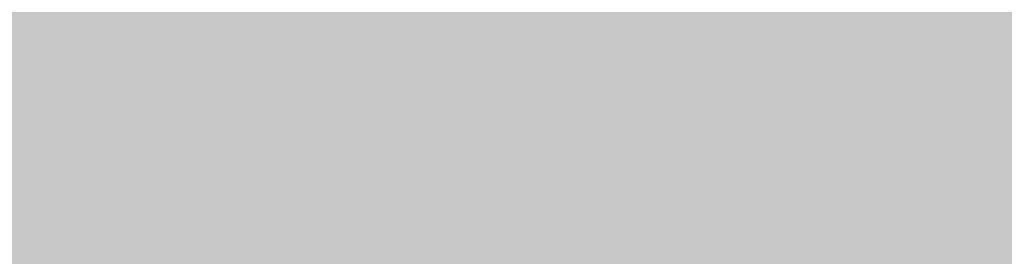
# Model space of a CAD drawing. Units: inches. Extents: x 2083 to 3317, y 1141 to 2115.
# Tile 135 of 256: x 3123.979 to 3126.132, y 1263.613 to 1264.131. Entities that reach past the tile are written whole.
import ezdxf

# ---------------------------------------------------------------- set-up
doc = ezdxf.new("R2010")
doc.units = ezdxf.units.IN
doc.layers.add('A-ANNO-DIMS', color=2, linetype='Continuous', lineweight=18)
doc.layers.add('A-WALL-PATT', color=251, linetype='Continuous', lineweight=13, true_color=0x636466)
doc.styles.get("Standard").update_dxf_attribs({"font": 'arial.ttf'})
doc.dimstyles.new('ISO-25', dxfattribs={"dimtxt": 12, "dimasz": 12, "dimexe": 1.25, "dimexo": 0.625, "dimtad": 1, "dimlunit": 3, "dimtxsty": 'Standard', "dimcen": 2.5, "dimadec": 0, "dimazin": 0, "dimtfac": 1, "dimtmove": 0, "dimatfit": 3, "dimfxl": 1, "dimarcsym": 0})

# ---------------------------------------------------------------- blocks, each defined once
blk = doc.blocks.new('*D26')
at = {"layer": 'A-ANNO-DIMS', "color": 0, "lineweight": -2, "transparency": 16777216}
for p, q in [((3088.9858, 1274.9151), (3088.9858, 1270.952)), ((3111.24, 1274.9151), (3111.24, 1270.952)), ((3076.9858, 1272.202), (2840.2624, 1272.202)), ((3111.24, 1272.202), (3088.9858, 1272.202)), ((3123.24, 1272.202), (3135.24, 1272.202))]:
    blk.add_line(p, q, dxfattribs=at)
at = {"layer": 'A-ANNO-DIMS', "color": 0, "transparency": 16777216}
for points in [[(3076.9858, 1274.202), (3076.9858, 1270.202), (3088.9858, 1272.202)], [(3123.24, 1274.202), (3123.24, 1270.202), (3111.24, 1272.202)]]:
    blk.add_solid(points, dxfattribs=at)
at = {"layer": 'Defpoints', "color": 0, "transparency": 16777216}
for p in [(3088.9858, 1275.5401), (3111.24, 1275.5401), (3088.9858, 1272.202)]:
    blk.add_point(p, dxfattribs=at)
at = {"layer": 'A-ANNO-DIMS', "color": 0, "transparency": 16777216, "insert": (2952.6241, 1279.0316), "char_height": 12, "attachment_point": 5}
blk.add_mtext('NIGHTSTAND 1\'-10 1/2" TYP.', dxfattribs=at)
blk = doc.blocks.new('*D27')
at = {"layer": 'A-ANNO-DIMS', "color": 0, "lineweight": -2, "transparency": 16777216}
for p, q in [((3114.5782, 1309.7943), (3114.5782, 1321.7943)), ((3111.865, 1297.7943), (3115.8282, 1297.7943)), ((3114.5782, 1297.7943), (3114.5782, 1275.5401)), ((3111.865, 1275.5401), (3115.8282, 1275.5401)), ((3114.5782, 1263.5401), (3114.5782, 1140.9886))]:
    blk.add_line(p, q, dxfattribs=at)
at = {"layer": 'A-ANNO-DIMS', "color": 0, "transparency": 16777216}
for points in [[(3112.5782, 1309.7943), (3116.5782, 1309.7943), (3114.5782, 1297.7943)], [(3112.5782, 1263.5401), (3116.5782, 1263.5401), (3114.5782, 1275.5401)]]:
    blk.add_solid(points, dxfattribs=at)
at = {"layer": 'Defpoints', "color": 0, "transparency": 16777216}
for p in [(3111.24, 1297.7943), (3111.24, 1275.5401), (3114.5782, 1275.5401)]:
    blk.add_point(p, dxfattribs=at)
at = {"layer": 'A-ANNO-DIMS', "color": 0, "transparency": 16777216, "insert": (3107.7485, 1196.2643), "char_height": 12, "attachment_point": 5, "rotation": 90}
blk.add_mtext('1\'-10 1/2" TYP.', dxfattribs=at)

msp = doc.modelspace()

# ---------------------------------------------------------------- hatches: boundary and pattern name
at = {"layer": 'A-WALL-PATT'}
h = msp.add_hatch(color=256, dxfattribs=at)
h.dxf.hatch_style = 1
h.paths.add_polyline_path([(3126.9598, 2020.7614), (2748.9598, 2020.7614), (2604.9598, 2020.7614), (2226.9598, 2020.7614), (2226.9598, 1702.7614), (2466.9598, 1702.7614), (2466.9598, 1582.7614), (2418.9598, 1582.7614), (2418.9598, 1477.7614), (2226.9598, 1477.7614), (2226.9598, 1263.2614), (2544.9598, 1263.2614), (2544.9598, 1411.7614), (2604.9598, 1411.7614), (2685.9598, 1411.7614), (2685.9598, 1420.7614), (2604.9598, 1420.7614), (2604.9598, 1573.7614), (2604.9598, 1702.7614), (2604.9598, 2011.7614), (2748.9598, 2011.7614), (2748.9598, 1702.7614), (2862.9598, 1702.7614), (2862.9598, 1621.7614), (2871.9598, 1621.7614), (2871.9598, 1702.7614), (2883.9598, 1702.7614), (2883.9598, 1706.9395, -0.026459), (2883.9598, 1711.7614), (2757.9598, 1711.7614), (2757.9598, 1807.7614), (2787.9598, 1807.7614), (2787.9598, 1812.2614), (2757.9598, 1812.2614), (2757.9598, 2011.7614), (2877.9598, 2011.7614), (2877.9598, 1812.2614), (2847.9598, 1812.2614), (2847.9598, 1807.7614), (2889.8357, 1807.7614), (2889.8357, 1812.2614), (2882.4598, 1812.2614), (2882.4598, 2011.7614), (3117.9598, 2011.7614), (3117.9598, 1812.2614), (2937.8357, 1812.2614), (2937.8357, 1807.7614), (2995.7098, 1807.7614), (2995.7098, 1796.1177), (3000.2098, 1796.1177), (3000.2098, 1807.7614), (3117.9598, 1807.7614), (3117.9598, 1711.7614), (3000.2098, 1711.7614), (3000.2098, 1760.1177), (2998.5727, 1760.1177, -0.020711), (2995.7098, 1760.1177), (2995.7098, 1711.7614), (2931.9598, 1711.7614), (2931.9598, 1702.7614), (3126.9598, 1702.7614)])
h.paths.add_polyline_path([(2471.4598, 2011.7614), (2471.4598, 1810.0114), (2462.7169, 1810.0114), (2462.7169, 1805.5114), (2505.9598, 1805.5114), (2505.9598, 1810.0114), (2475.9598, 1810.0114), (2475.9598, 2011.7614), (2595.9598, 2011.7614), (2595.9598, 1810.0114), (2565.9598, 1810.0114), (2565.9598, 1805.5114), (2595.9598, 1805.5114), (2595.9598, 1711.7614), (2235.9598, 1711.7614), (2235.9598, 1805.5114), (2353.7098, 1805.5114), (2353.7098, 1796.0542), (2358.2098, 1796.0542), (2358.2098, 1805.5114), (2414.7169, 1805.5114), (2414.7169, 1810.0114), (2235.9598, 1810.0114), (2235.9598, 2011.7614)], flags=16)
h.paths.add_polyline_path([(2270.2047, 1994.61), (2270.2047, 1970.61), (2246.2047, 1970.61), (2246.2047, 1994.61)], flags=0)
edge = h.paths.add_edge_path(flags=0)
edge.add_ellipse((2332.0274, 1899.7982), major_axis=(-3.043, 3.043), ratio=0.168252, start_angle=-161.3322, end_angle=-156.3071, ccw=False)
edge.add_ellipse((2333.082, 1898.7435), major_axis=(-1.0546, 1.0546), ratio=0.453532, start_angle=-123.371, end_angle=-94.1591)
edge = h.paths.add_edge_path(flags=0)
edge.add_ellipse((2332.0274, 1968.8763), major_axis=(3.043, 3.043), ratio=0.168252, start_angle=18.6678, end_angle=23.6929)
edge.add_spline(control_points=[(2332.9256, 1970.6911), (2332.2268, 1970.3361), (2330.8937, 1969.6589), (2328.4131, 1970.9321), (2327.2039, 1967.7487), (2324.7096, 1969.9556), (2322.5328, 1967.0124), (2320.0128, 1971.2958), (2317.6803, 1968.1578), (2316.0405, 1967.102), (2315.4269, 1966.8096)], knot_values=[0, 0, 0, 0, 2.267059, 4.324559, 6.685584, 8.878641, 11.121502, 14.300359, 17.755284, 19.732645, 19.732645, 19.732645, 19.732645], degree=3, periodic=0)
edge.add_ellipse((2332.0274, 1968.8763), major_axis=(3.043, 3.043), ratio=0.168252, start_angle=18.6678, end_angle=23.6929, ccw=False)
edge.add_ellipse((2333.082, 1969.9309), major_axis=(1.0546, 1.0546), ratio=0.453532, start_angle=56.629, end_angle=85.8409, ccw=False)
edge = h.paths.add_edge_path(flags=0)
edge.add_spline(control_points=[(2296.4283, 1967.9879), (2293.6278, 1965.3363), (2287.7036, 1959.7271), (2299.7439, 1949.9957), (2294.5326, 1935.6685), (2290.5732, 1920.6035), (2293.3941, 1909.9737), (2296.1854, 1904.9665)], knot_values=[0.099185, 0.099185, 0.099185, 0.099185, 0.345301, 0.619822, 0.982653, 1.386093, 1.810555, 1.810555, 1.810555, 1.810555], degree=3, periodic=0)
edge.add_spline(control_points=[(2296.1854, 1904.9665), (2297.3836, 1902.6193), (2298.001, 1901.9493), (2298.553, 1901.4682)], knot_values=[0.006246, 0.006246, 0.006246, 0.006246, 0.055476, 0.055476, 0.055476, 0.055476], degree=3, periodic=0)
edge.add_spline(control_points=[(2298.553, 1901.4682), (2297.2586, 1900.9232), (2295.2253, 1900.2321), (2293.0602, 1900.6142), (2292.1014, 1900.7884), (2292.0896, 1900.7906)], knot_values=[0.312835, 0.312835, 0.312835, 0.312835, 0.40178, 0.474987, 0.475903, 0.475903, 0.475903, 0.475903], degree=3, periodic=0)
edge.add_arc((2292.7936, 1904.6641), 3.937, 215.4209, 259.6982, ccw=False)
edge.add_spline(control_points=[(2289.5853, 1902.3823), (2289.4767, 1902.5351), (2289.3685, 1902.688), (2289.2609, 1902.8412)], knot_values=[0.102872, 0.102872, 0.102872, 0.102872, 0.116896, 0.116896, 0.116896, 0.116896], degree=3, periodic=0)
edge.add_spline(control_points=[(2289.2609, 1902.8412), (2288.6866, 1902.5502), (2287.64, 1902.0199), (2285.8813, 1901.874), (2283.853, 1901.5044), (2281.72, 1899.7105), (2278.467, 1899.4929), (2276.1571, 1901.8832), (2272.259, 1899.8041), (2267.7776, 1901.8432), (2262.2439, 1900.184), (2257.4149, 1901.7821), (2254.3184, 1900.7261), (2253.1783, 1900.3373)], knot_values=[0, 0, 0, 0, 1.907977, 3.477176, 5.261074, 7.972851, 11.680248, 13.717921, 16.939592, 22.789562, 27.502503, 33.595215, 37.145618, 37.145618, 37.145618, 37.145618], degree=3, periodic=0)
edge.add_line((2253.1783, 1900.3373), (2250.2442, 1902.8412))
edge.add_line((2250.2442, 1902.8412), (2250.2442, 1965.8333))
edge.add_line((2250.2442, 1965.8333), (2253.1783, 1968.3371))
edge.add_spline(control_points=[(2253.1783, 1968.3371), (2254.3184, 1967.9483), (2257.4149, 1966.8924), (2262.2439, 1968.4904), (2267.7776, 1966.8313), (2271.5267, 1968.5372), (2273.8759, 1967.8283), (2274.2067, 1967.7276)], knot_values=[0, 0, 0, 0, 0.09018, 0.244935, 0.364644, 0.513233, 0.537855, 0.537855, 0.537855, 0.537855], degree=3, periodic=0)
edge.add_arc((2274.3529, 1963.7933), 3.937, 72.0511, 92.1279, ccw=False)
edge.add_arc((2281.2969, 1985.23), 18.5963, 252.05113, 288.56572)
edge.add_arc((2292.3167, 1956.0289), 12.6461, 71.02679, 113.77822, ccw=False)
edge = h.paths.add_edge_path(flags=0)
edge.add_spline(control_points=[(2274.8994, 1951.8562), (2275.0662, 1951.6166), (2275.2327, 1951.3766), (2275.398, 1951.1359)], knot_values=[1.409916, 1.409916, 1.409916, 1.409916, 1.43159, 1.43159, 1.43159, 1.43159], degree=3, periodic=0)
edge.add_spline(control_points=[(2275.398, 1951.1359), (2275.7921, 1950.5619), (2276.1792, 1949.9838), (2276.5455, 1949.3971)], knot_values=[1.358238, 1.358238, 1.358238, 1.358238, 1.409916, 1.409916, 1.409916, 1.409916], degree=3, periodic=0)
edge.add_line((2276.5455, 1949.3971), (2277.4373, 1947.8622))
edge.add_spline(control_points=[(2277.4373, 1947.8622), (2276.3038, 1945.6731), (2274.6397, 1942.4269), (2274.6316, 1938.0939), (2272.7991, 1930.8515), (2274.3564, 1943.897), (2275.9477, 1947.9234), (2276.5455, 1949.3971)], knot_values=[0.005632, 0.005632, 0.005632, 0.005632, 0.186014, 0.266002, 0.357087, 0.59639, 0.739732, 0.739732, 0.739732, 0.739732], degree=3, periodic=0)
edge.add_spline(control_points=[(2276.5455, 1949.3971), (2276.1792, 1949.9838), (2275.7921, 1950.5619), (2275.398, 1951.1359)], knot_values=[1.358238, 1.358238, 1.358238, 1.358238, 1.409916, 1.409916, 1.409916, 1.409916], degree=3, periodic=0)
edge.add_spline(control_points=[(2275.398, 1951.1359), (2274.9425, 1950.0805), (2274.2078, 1948.0253), (2273.9346, 1944.8515), (2272.4685, 1937.6275), (2273.4662, 1945.6965), (2274.7006, 1951.0595), (2274.8994, 1951.8562)], knot_values=[0.104364, 0.104364, 0.104364, 0.104364, 0.189636, 0.269624, 0.36071, 0.600013, 0.644622, 0.644622, 0.644622, 0.644622], degree=3, periodic=0)
h.paths.add_polyline_path([(2269.1675, 1963.1276, -0.357527), (2268.1706, 1960.9764, -0.092561), (2268.1706, 1939.4363, -0.357527), (2269.1675, 1937.2851, -0.357527), (2267.0163, 1938.282, -0.164785), (2254.6856, 1938.282, -0.357527), (2252.5344, 1937.2851, -0.357527), (2253.5313, 1939.4363, -0.092561), (2253.5313, 1960.9764, -0.357527), (2252.5344, 1963.1276, -0.357527), (2254.6856, 1962.1307, -0.164785), (2267.0163, 1962.1307, -0.357527)], flags=0)
h.paths.add_polyline_path([(2248.8741, 1967.8018), (2248.8741, 1957.0277), (2249.4578, 1957.0277), (2249.4578, 1911.6468), (2248.8741, 1911.6468), (2248.8741, 1900.8727), (2246.5119, 1900.8727, 0.197327), (2244.1497, 1902.4569), (2244.1497, 1966.2176, 0.197327), (2246.5119, 1967.8018)], flags=0)
h.paths.add_polyline_path([(2269.1675, 1931.3893, -0.357527), (2268.1706, 1929.2381, -0.092561), (2268.1706, 1907.6981, -0.357527), (2269.1675, 1905.5469, -0.357527), (2267.0163, 1906.5438, -0.164785), (2254.6856, 1906.5438, -0.357527), (2252.5344, 1905.5469, -0.357527), (2253.5313, 1907.6981, -0.092561), (2253.5313, 1929.2381, -0.357527), (2252.5344, 1931.3893, -0.357527), (2254.6856, 1930.3925, -0.164785), (2267.0163, 1930.3925, -0.357527)], flags=0)
edge = h.paths.add_edge_path(flags=0)
edge.add_spline(control_points=[(2276.1969, 1906.7237), (2276.1681, 1909.0289), (2276.114, 1913.3719), (2270.5984, 1924.925), (2273.9052, 1919.0128), (2275.9217, 1916.2621), (2275.4746, 1912.4021), (2277.2579, 1910.3806), (2276.696, 1908.225), (2276.6462, 1906.813), (2276.6178, 1906.0084)], knot_values=[0, 0, 0, 0, 8.61026, 16.221274, 18.843057, 23.804898, 27.440828, 29.356102, 31.203478, 33.650687, 33.650687, 33.650687, 33.650687], degree=3, periodic=0)
edge.add_spline(control_points=[(2276.6178, 1906.0084), (2276.6233, 1905.6241), (2276.4977, 1904.6287), (2275.4418, 1903.8547), (2274.9373, 1903.0804), (2274.8591, 1902.8412)], knot_values=[0.156488, 0.156488, 0.156488, 0.156488, 0.184398, 0.231376, 0.250598, 0.250598, 0.250598, 0.250598], degree=3, periodic=0)
edge.add_line((2274.8591, 1902.8412), (2276.506, 1902.8412))
edge.add_spline(control_points=[(2276.506, 1902.8412), (2276.7883, 1903.0849), (2277.6651, 1904.1252), (2278.2495, 1904.3407), (2277.6539, 1908.5274), (2278.1557, 1906.2278), (2278.1005, 1905.2859), (2278.8467, 1904.069), (2277.8568, 1903.4149), (2277.8742, 1902.991), (2277.9036, 1902.8412)], knot_values=[0.059574, 0.059574, 0.059574, 0.059574, 0.080753, 0.103741, 0.16972, 0.176036, 0.207137, 0.240474, 0.262341, 0.27366, 0.27366, 0.27366, 0.27366], degree=3, periodic=0)
edge.add_line((2277.9036, 1902.8412), (2280.0298, 1902.8412))
edge.add_spline(control_points=[(2280.0298, 1902.8412), (2279.8882, 1903.0884), (2279.4993, 1903.9816), (2280.1523, 1905.9393), (2278.1036, 1909.6578), (2279.7624, 1907.1853), (2280.3279, 1904.8749), (2280.4851, 1903.4896), (2281.4633, 1903.2494), (2281.7583, 1902.9365), (2281.834, 1902.8412)], knot_values=[0.013856, 0.013856, 0.013856, 0.013856, 0.034874, 0.088867, 0.107879, 0.126738, 0.158714, 0.193757, 0.217487, 0.226722, 0.226722, 0.226722, 0.226722], degree=3, periodic=0)
edge.add_spline(control_points=[(2281.834, 1902.8412), (2281.7875, 1902.8267), (2281.647, 1902.783), (2281.3955, 1902.8595), (2281.0881, 1902.9852), (2280.7207, 1903.0609), (2280.3335, 1903.0257), (2280.1248, 1902.8989), (2280.0298, 1902.8412)], knot_values=[0, 0, 0, 0, 0.14413, 0.435517, 0.749276, 1.153046, 1.548371, 1.878348, 1.878348, 1.878348, 1.878348], degree=3, periodic=0)
edge.add_line((2280.0298, 1902.8412), (2277.9036, 1902.8412))
edge.add_spline(control_points=[(2277.9036, 1902.8412), (2277.8929, 1902.7959), (2277.8654, 1902.6796), (2277.6075, 1902.6875), (2277.2741, 1902.8007), (2276.8379, 1902.6198), (2276.5838, 1902.7893), (2276.506, 1902.8412)], knot_values=[0, 0, 0, 0, 0.127189, 0.326199, 0.628009, 1.24357, 1.515331, 1.515331, 1.515331, 1.515331], degree=3, periodic=0)
edge.add_line((2276.506, 1902.8412), (2274.8591, 1902.8412))
edge.add_spline(control_points=[(2274.8591, 1902.8412), (2274.8144, 1902.8986), (2274.7251, 1903.0134), (2274.4935, 1903.119), (2274.2443, 1902.9605), (2273.9371, 1903.1849), (2273.614, 1902.9831), (2273.4083, 1902.883), (2273.3223, 1902.8412)], knot_values=[0, 0, 0, 0, 0.21843, 0.436957, 0.687977, 0.990379, 1.398396, 1.69185, 1.69185, 1.69185, 1.69185], degree=3, periodic=0)
edge.add_spline(control_points=[(2273.3223, 1902.8412), (2273.6167, 1903.4457), (2274.274, 1904.5383), (2276.0272, 1904.5737), (2276.207, 1906.5836), (2276.1969, 1906.7237)], knot_values=[0.012227, 0.012227, 0.012227, 0.012227, 0.059472, 0.106218, 0.134458, 0.134458, 0.134458, 0.134458], degree=3, periodic=0)
h.paths.add_polyline_path([(2270.7761, 1897.7898), (2270.7761, 1873.7898), (2246.7761, 1873.7898), (2246.7761, 1897.7898)], flags=0)
h.paths.add_polyline_path([(2353.7098, 1760.0051), (2353.7098, 1760.0542), (2358.2098, 1760.0542, -0.033729)], flags=0)
h.paths.add_polyline_path([(2321.8191, 1737.5292), (2341.9953, 1737.5292, -0.414214), (2343.2033, 1736.3212), (2343.2033, 1721.0206, -0.414214), (2341.9953, 1719.8127), (2321.8191, 1719.8127, -0.414214), (2320.6112, 1721.0206), (2320.6112, 1736.3212, -0.414214)], flags=0)
h.paths.add_polyline_path([(2324.235, 1736.3212), (2339.5794, 1736.3212, -0.414214), (2341.9953, 1733.9053), (2341.9953, 1725.4497, -0.414214), (2339.5794, 1723.0338), (2333.6806, 1723.0338), (2333.8453, 1722.0455, -0.870646), (2335.4254, 1721.8259, -0.767327), (2333.9227, 1721.4232), (2331.291, 1721.4232, -0.767327), (2329.7883, 1721.8259, -0.870646), (2331.3684, 1722.0455), (2331.5331, 1723.0338), (2324.235, 1723.0338, -0.414214), (2321.8191, 1725.4497), (2321.8191, 1733.9053, -0.414214)], flags=0)
h.paths.add_polyline_path([(2570.4838, 1928.6154), (2589.6838, 1928.6154), (2590.1688, 1928.6154), (2590.1688, 1904.9934), (2570.4838, 1904.9934)], flags=0)
h.paths.add_polyline_path([(2574.4473, 1927.2638, -1), (2572.8288, 1927.2638, -1)], flags=0)
h.paths.add_polyline_path([(2573.0899, 1926.9409), (2573.925, 1927.776), (2574.1477, 1927.5533), (2573.3126, 1926.7182)], flags=0)
h.paths.add_polyline_path([(2578.7791, 1919.7296, -1), (2571.5917, 1919.7296, -1)], flags=0)
h.paths.add_polyline_path([(2578.3854, 1919.7296, -1), (2571.9854, 1919.7296, -1)], flags=0)
h.paths.add_polyline_path([(2331.5958, 1729.4762, -1), (2333.618, 1729.4762, -1)], flags=0)
h.paths.add_polyline_path([(2578.0342, 1927.2638, -1), (2576.4157, 1927.2638, -1)], flags=0)
h.paths.add_polyline_path([(2576.6889, 1927.5311), (2576.9116, 1927.7538), (2577.7467, 1926.9186), (2577.524, 1926.6959)], flags=0)
h.paths.add_polyline_path([(2578.1391, 1909.8595, -1), (2572.2317, 1909.8595, -1)], flags=0)
h.paths.add_polyline_path([(2577.7454, 1909.8595, -1), (2572.6254, 1909.8595, -1)], flags=0)
h.paths.add_polyline_path([(2583.7977, 1927.2638, -1), (2582.1792, 1927.2638, -1)], flags=0)
h.paths.add_polyline_path([(2582.7186, 1927.7538), (2583.5538, 1926.9186), (2583.3311, 1926.6959), (2582.4959, 1927.5311)], flags=0)
h.paths.add_polyline_path([(2582.4959, 1927.5311), (2582.7186, 1927.7538), (2583.5538, 1926.9186), (2583.3311, 1926.6959)], flags=0)
h.paths.add_polyline_path([(2587.7391, 1920.5296, -1), (2581.8317, 1920.5296, -1)], flags=0)
h.paths.add_polyline_path([(2587.3454, 1920.5296, -1), (2582.2254, 1920.5296, -1)], flags=0)
h.paths.add_polyline_path([(2587.3846, 1927.2638, -1), (2585.7661, 1927.2638, -1)], flags=0)
h.paths.add_polyline_path([(2586.082, 1926.9802), (2586.9172, 1927.8154), (2587.1399, 1927.5927), (2586.3047, 1926.7575)], flags=0)
h.paths.add_polyline_path([(2588.3791, 1910.6595, -1), (2581.1917, 1910.6595, -1)], flags=0)
h.paths.add_polyline_path([(2587.9854, 1910.6595, -1), (2581.5854, 1910.6595, -1)], flags=0)
h.paths.add_polyline_path([(2417.1677, 1729.4779), (2437.3439, 1729.4779, -0.414214), (2438.5519, 1728.2699), (2438.5519, 1712.9693, -0.414214), (2437.3439, 1711.7614), (2417.1677, 1711.7614, -0.414214), (2415.9598, 1712.9693), (2415.9598, 1728.2699, -0.414214)], flags=0)
h.paths.add_polyline_path([(2419.5836, 1728.2699), (2434.928, 1728.2699, -0.414214), (2437.3439, 1725.8541), (2437.3439, 1717.3984, -0.414214), (2434.928, 1714.9825), (2429.0292, 1714.9825), (2429.1939, 1713.9942, -0.870646), (2430.774, 1713.7746, -0.767327), (2429.2713, 1713.372), (2426.6396, 1713.372, -0.767327), (2425.1369, 1713.7746, -0.870646), (2426.717, 1713.9942), (2426.8817, 1714.9825), (2419.5836, 1714.9825, -0.414214), (2417.1677, 1717.3984), (2417.1677, 1725.8541, -0.414214)], flags=0)
h.paths.add_polyline_path([(2419.5836, 1728.2699), (2434.928, 1728.2699, -0.414214), (2437.3439, 1725.8541), (2437.3439, 1717.3984, -0.414214), (2434.928, 1714.9825), (2429.0292, 1714.9825), (2428.3581, 1719.009), (2427.5528, 1719.009), (2426.8817, 1714.9825), (2419.5836, 1714.9825, -0.414214), (2417.1677, 1717.3984), (2417.1677, 1725.8541, -0.414214)], flags=0)
h.paths.add_polyline_path([(2426.9444, 1721.4249, -1), (2428.9666, 1721.4249, -1)], flags=0)
h.paths.add_polyline_path([(2475.9598, 1702.7614), (2595.9598, 1702.7614), (2595.9598, 1582.7614), (2475.9598, 1582.7614)], flags=16)
h.paths.add_polyline_path([(2427.9598, 1573.7614), (2595.9598, 1573.7614), (2595.9598, 1468.7614), (2595.9598, 1420.7614), (2384.4598, 1420.7614), (2384.4598, 1468.7614), (2427.9598, 1468.7614)], flags=16)
h.paths.add_polyline_path([(2379.9598, 1468.7614), (2379.9598, 1420.7614), (2235.9598, 1420.7614), (2235.9598, 1468.7614)], flags=16)
h.paths.add_polyline_path([(2317.816, 1466.6958), (2337.9922, 1466.6958, -0.414214), (2339.2002, 1465.4878), (2339.2002, 1450.1872, -0.414214), (2337.9922, 1448.9792), (2317.816, 1448.9792, -0.414214), (2316.6081, 1450.1872), (2316.6081, 1465.4878, -0.414214)], flags=0)
h.paths.add_polyline_path([(2320.2319, 1465.4878), (2335.5763, 1465.4878, -0.414214), (2337.9922, 1463.0719), (2337.9922, 1454.6163, -0.414214), (2335.5763, 1452.2004), (2329.6775, 1452.2004), (2329.8422, 1451.212, -0.870646), (2331.4223, 1450.9925, -0.767327), (2329.9196, 1450.5898), (2327.2879, 1450.5898, -0.767327), (2325.7852, 1450.9925, -0.870646), (2327.3653, 1451.212), (2327.53, 1452.2004), (2320.2319, 1452.2004, -0.414214), (2317.816, 1454.6163), (2317.816, 1463.0719, -0.414214)], flags=0)
h.paths.add_polyline_path([(2320.2319, 1465.4878), (2335.5763, 1465.4878, -0.414214), (2337.9922, 1463.0719), (2337.9922, 1454.6163, -0.414214), (2335.5763, 1452.2004), (2329.6775, 1452.2004), (2329.0064, 1456.2269), (2328.2011, 1456.2269), (2327.53, 1452.2004), (2320.2319, 1452.2004, -0.414214), (2317.816, 1454.6163), (2317.816, 1463.0719, -0.414214)], flags=0)
h.paths.add_polyline_path([(2327.5926, 1458.6428, -1), (2329.6148, 1458.6428, -1)], flags=0)
h.paths.add_polyline_path([(2244.4117, 1433.3405), (2241.9209, 1433.3405, -0.414214), (2240.0179, 1435.2435), (2240.0179, 1440.9528, -0.414211), (2241.9209, 1442.8559), (2244.4117, 1442.8559, -1.976472)], flags=0)
h.paths.add_polyline_path([(2245.3569, 1434.3975, -0.414214), (2245.3569, 1441.7988, -2.144098)], flags=0)
h.paths.add_polyline_path([(2535.9598, 1416.2614), (2535.9598, 1272.2614), (2235.9598, 1272.2614), (2235.9598, 1416.2614)], flags=16)
h.paths.add_polyline_path([(2260.1196, 1384.2928), (2260.1196, 1362.0386), (2237.8654, 1362.0386), (2237.8654, 1384.2928)], flags=0)
edge = h.paths.add_edge_path(flags=0)
edge.add_line((2318.2518, 1362.0933), (2318.1458, 1362.001))
edge.add_ellipse((2317.4451, 1360.431), major_axis=(2.8216, 2.8216), ratio=0.168252, start_angle=18.6678, end_angle=20.9481, ccw=False)
edge.add_ellipse((2318.423, 1361.409), major_axis=(0.9779, 0.9779), ratio=0.453532, start_angle=56.629, end_angle=70.2262, ccw=False)
edge = h.paths.add_edge_path(flags=0)
edge.add_line((2319.1074, 1295.5711), (2319.015, 1295.6771))
edge.add_ellipse((2317.4451, 1296.3778), major_axis=(-2.8216, 2.8216), ratio=0.168252, start_angle=-161.3322, end_angle=-159.0519, ccw=False)
edge.add_ellipse((2318.423, 1295.3999), major_axis=(-0.9779, 0.9779), ratio=0.453532, start_angle=-123.371, end_angle=-109.7738)
edge = h.paths.add_edge_path(flags=0)
edge.add_spline(control_points=[(2284.2103, 1301.1702), (2284.5807, 1300.4447), (2284.8912, 1299.892), (2285.1596, 1299.461)], knot_values=[0.039066, 0.039066, 0.039066, 0.039066, 0.055476, 0.055476, 0.055476, 0.055476], degree=3, periodic=0)
edge.add_line((2285.1596, 1299.461), (2284.2103, 1301.1702))
edge = h.paths.add_edge_path(flags=0)
edge.add_line((2280.4125, 1297.298), (2283.37, 1297.0361))
edge.add_line((2283.37, 1297.0361), (2286.4057, 1297.9263))
edge.add_spline(control_points=[(2286.4057, 1297.9263), (2285.3055, 1297.4631), (2284.3448, 1297.1292), (2283.37, 1297.0361)], knot_values=[0.394369, 0.394369, 0.394369, 0.394369, 0.475903, 0.475903, 0.475903, 0.475903], degree=3, periodic=0)
edge.add_spline(control_points=[(2283.37, 1297.0361), (2283.2814, 1297.0277), (2282.3163, 1296.9573), (2281.3125, 1297.1345), (2280.4234, 1297.296), (2280.4125, 1297.298)], knot_values=[0.312835, 0.312835, 0.312835, 0.312835, 0.320246, 0.393453, 0.394369, 0.394369, 0.394369, 0.394369], degree=3, periodic=0)
edge = h.paths.add_edge_path(flags=0)
edge.add_line((2284.4356, 1359.6073), (2280.4463, 1355.328))
edge.add_line((2280.4463, 1355.328), (2279.58, 1351.0178))
edge.add_line((2279.58, 1351.0178), (2282.413, 1346.5804))
edge.add_spline(control_points=[(2282.413, 1346.5804), (2283.1533, 1345.5892), (2284.2529, 1344.0289), (2284.801, 1342.3872), (2284.9352, 1341.8055)], knot_values=[1.240098, 1.240098, 1.240098, 1.240098, 1.332892, 1.382712, 1.382712, 1.382712, 1.382712], degree=3, periodic=0)
edge.add_spline(control_points=[(2284.9352, 1341.8055), (2285.3191, 1340.1406), (2285.233, 1338.4092), (2284.9099, 1336.6541)], knot_values=[1.097484, 1.097484, 1.097484, 1.097484, 1.240098, 1.240098, 1.240098, 1.240098], degree=3, periodic=0)
edge.add_spline(control_points=[(2284.9099, 1336.6541), (2284.5868, 1334.899), (2284.0267, 1333.1203), (2283.4626, 1331.3606)], knot_values=[0.95487, 0.95487, 0.95487, 0.95487, 1.097484, 1.097484, 1.097484, 1.097484], degree=3, periodic=0)
edge.add_line((2283.4626, 1331.3606), (2281.8904, 1326.1534))
edge.add_line((2281.8904, 1326.1534), (2280.7563, 1321.0561))
edge.add_line((2280.7563, 1321.0561), (2280.2992, 1316.002))
edge.add_line((2280.2992, 1316.002), (2280.7159, 1310.9501))
edge.add_line((2280.7159, 1310.9501), (2282.0281, 1305.9721))
edge.add_line((2282.0281, 1305.9721), (2284.2103, 1301.1702))
edge.add_spline(control_points=[(2284.2103, 1301.1702), (2283.3407, 1302.7302), (2282.6119, 1304.3365), (2282.0281, 1305.9721)], knot_values=[0.099185, 0.099185, 0.099185, 0.099185, 0.241799, 0.241799, 0.241799, 0.241799], degree=3, periodic=0)
edge.add_spline(control_points=[(2282.0281, 1305.9721), (2281.4443, 1307.6078), (2281.0055, 1309.2728), (2280.7159, 1310.9501)], knot_values=[0.241799, 0.241799, 0.241799, 0.241799, 0.384413, 0.384413, 0.384413, 0.384413], degree=3, periodic=0)
edge.add_spline(control_points=[(2280.7159, 1310.9501), (2280.4332, 1312.5876), (2280.2894, 1314.277), (2280.2989, 1315.962), (2280.2992, 1316.002)], knot_values=[0.384413, 0.384413, 0.384413, 0.384413, 0.523647, 0.527028, 0.527028, 0.527028, 0.527028], degree=3, periodic=0)
edge.add_spline(control_points=[(2280.2992, 1316.002), (2280.3123, 1317.687), (2280.4779, 1319.3679), (2280.7563, 1321.0561)], knot_values=[0.527028, 0.527028, 0.527028, 0.527028, 0.669642, 0.669642, 0.669642, 0.669642], degree=3, periodic=0)
edge.add_spline(control_points=[(2280.7563, 1321.0561), (2281.0346, 1322.7443), (2281.4259, 1324.4396), (2281.8904, 1326.1534)], knot_values=[0.669642, 0.669642, 0.669642, 0.669642, 0.812256, 0.812256, 0.812256, 0.812256], degree=3, periodic=0)
edge.add_spline(control_points=[(2281.8904, 1326.1534), (2282.2644, 1327.5333), (2282.7879, 1329.2618), (2283.3528, 1331.0178), (2283.4626, 1331.3606)], knot_values=[0.812256, 0.812256, 0.812256, 0.812256, 0.927087, 0.95487, 0.95487, 0.95487, 0.95487], degree=3, periodic=0)
edge.add_line((2283.4626, 1331.3606), (2284.9099, 1336.6541))
edge.add_line((2284.9099, 1336.6541), (2284.9352, 1341.8055))
edge.add_line((2284.9352, 1341.8055), (2282.413, 1346.5804))
edge.add_spline(control_points=[(2282.413, 1346.5804), (2281.2751, 1348.1038), (2280.0784, 1349.5703), (2279.58, 1351.0178)], knot_values=[1.382712, 1.382712, 1.382712, 1.382712, 1.525326, 1.525326, 1.525326, 1.525326], degree=3, periodic=0)
edge.add_spline(control_points=[(2279.58, 1351.0178), (2279.4433, 1351.4147), (2279.1363, 1352.8569), (2279.7352, 1354.2904), (2280.4463, 1355.328)], knot_values=[1.525326, 1.525326, 1.525326, 1.525326, 1.564439, 1.667941, 1.667941, 1.667941, 1.667941], degree=3, periodic=0)
edge.add_spline(control_points=[(2280.4463, 1355.328), (2281.4261, 1356.7578), (2282.9308, 1358.1826), (2284.4356, 1359.6073)], knot_values=[1.667941, 1.667941, 1.667941, 1.667941, 1.810555, 1.810555, 1.810555, 1.810555], degree=3, periodic=0)
edge.add_arc((2280.6231, 1348.5182), 11.7262, 71.02679, 113.77822)
edge.add_arc((2270.4049, 1375.5952), 17.2436, 252.05113, 288.56572, ccw=False)
edge.add_arc((2263.966, 1355.7178), 3.6506, 72.0511, 92.1279)
edge.add_arc((2263.966, 1355.7178), 3.6506, 92.1279, 177.9851)
edge.add_spline(control_points=[(2260.3176, 1355.8462), (2260.2604, 1354.2207), (2260.5513, 1350.1865), (2262.9993, 1346.7663), (2264.4727, 1344.649)], knot_values=[1.43159, 1.43159, 1.43159, 1.43159, 1.564144, 1.770695, 1.770695, 1.770695, 1.770695], degree=3, periodic=0)
edge.add_line((2264.4727, 1344.649), (2264.9356, 1343.9825))
edge.add_spline(control_points=[(2263.801, 1340.2481), (2263.8432, 1340.5141), (2264.0672, 1341.7565), (2264.5127, 1343.0025), (2264.935, 1343.9811)], knot_values=[0.53657, 0.53657, 0.53657, 0.53657, 0.559349, 0.644622, 0.644622, 0.644622, 0.644622], degree=3, periodic=0)
edge.add_spline(control_points=[(2264.935, 1343.9811), (2265.1178, 1343.715), (2265.2989, 1343.4479), (2265.4768, 1343.1794)], knot_values=[1.384077, 1.384077, 1.384077, 1.384077, 1.409916, 1.409916, 1.409916, 1.409916], degree=3, periodic=0)
edge.add_spline(control_points=[(2265.4768, 1343.1794), (2265.6546, 1342.9108), (2265.8293, 1342.6408), (2265.9991, 1342.3688)], knot_values=[1.358238, 1.358238, 1.358238, 1.358238, 1.384077, 1.384077, 1.384077, 1.384077], degree=3, periodic=0)
edge.add_line((2265.9991, 1342.3688), (2266.826, 1340.9455))
edge.add_spline(control_points=[(2266.826, 1340.9455), (2268.8944, 1337.0897), (2271.3982, 1325.843), (2270.5162, 1310.5686), (2275.9194, 1301.8606), (2277.7895, 1299.1994)], knot_values=[0.116896, 0.116896, 0.116896, 0.116896, 0.472987, 1.050969, 1.313793, 1.313793, 1.313793, 1.313793], degree=3, periodic=0)
edge.add_spline(control_points=[(2277.7895, 1299.1994), (2277.8394, 1299.1285), (2277.8894, 1299.0575), (2277.9396, 1298.9866)], knot_values=[0.109884, 0.109884, 0.109884, 0.109884, 0.116896, 0.116896, 0.116896, 0.116896], degree=3, periodic=0)
edge.add_line((2277.9396, 1298.9866), (2277.7888, 1299.1991))
edge.add_spline(control_points=[(2277.7888, 1299.1991), (2277.2566, 1298.9294), (2276.2864, 1298.4379), (2275.0394, 1298.3344), (2274.3833, 1298.2389), (2274.2153, 1298.2093)], knot_values=[33.12187, 33.12187, 33.12187, 33.12187, 35.029056, 36.598255, 37.144827, 37.144827, 37.144827, 37.144827], degree=3, periodic=0)
edge.add_line((2274.2153, 1298.2093), (2273.0731, 1297.893))
edge.add_spline(control_points=[(2273.0731, 1297.893), (2272.3229, 1297.5798), (2271.0392, 1296.5105), (2269.2484, 1296.2261), (2268.4231, 1296.3747)], knot_values=[26.532584, 26.532584, 26.532584, 26.532584, 29.198919, 31.839101, 31.839101, 31.839101, 31.839101], degree=3, periodic=0)
edge.add_line((2268.4231, 1296.3747), (2263.8785, 1297.4575))
edge.add_spline(control_points=[(2263.8785, 1297.4575), (2263.5561, 1297.3594), (2261.8603, 1296.8387), (2260.2388, 1297.2824), (2258.9335, 1297.5165)], knot_values=[15.919551, 15.919551, 15.919551, 15.919551, 16.939592, 21.226067, 21.226067, 21.226067, 21.226067], degree=3, periodic=0)
edge.add_line((2258.9335, 1297.5165), (2254.0552, 1297.329))
edge.add_spline(control_points=[(2254.0552, 1297.329), (2253.7555, 1297.2958), (2252.1137, 1297.1652), (2250.4619, 1297.5442), (2249.1297, 1297.6679)], knot_values=[5.306517, 5.306517, 5.306517, 5.306517, 6.276435, 10.613034, 10.613034, 10.613034, 10.613034], degree=3, periodic=0)
edge.add_line((2249.1297, 1297.6679), (2244.3316, 1296.8778))
edge.add_line((2244.3316, 1296.8778), (2241.611, 1299.1994))
edge.add_line((2241.611, 1299.1994), (2241.611, 1357.6094))
edge.add_line((2241.611, 1357.6094), (2244.3316, 1359.9311))
edge.add_line((2244.3316, 1359.9311), (2252.7288, 1359.5427))
edge.add_spline(control_points=[(2252.7288, 1359.5427), (2252.8709, 1359.5464), (2253.3057, 1359.5482), (2253.7398, 1359.5143), (2254.0317, 1359.4824)], knot_values=[0.233291, 0.233291, 0.233291, 0.233291, 0.244935, 0.268927, 0.268927, 0.268927, 0.268927], degree=3, periodic=0)
edge.add_line((2254.0317, 1359.4824), (2259.5872, 1359.4164))
edge.add_spline(control_points=[(2259.5872, 1359.4164), (2260.6771, 1359.6285), (2262.0732, 1359.897), (2263.5237, 1359.4593), (2263.8304, 1359.366)], knot_values=[0.422516, 0.422516, 0.422516, 0.422516, 0.513233, 0.537855, 0.537855, 0.537855, 0.537855], degree=3, periodic=0)
edge.add_arc((2263.966, 1355.7178), 3.6506, 72.0511, 92.1279, ccw=False)
edge.add_arc((2270.4049, 1375.5952), 17.2436, 252.05113, 288.56572)
edge.add_arc((2280.6231, 1348.5182), 11.7262, 71.02679, 113.77822, ccw=False)
h.paths.add_polyline_path([(2240.3405, 1359.4347), (2240.3405, 1349.4444), (2240.8818, 1349.4444), (2240.8818, 1307.3645), (2240.3405, 1307.3645), (2240.3405, 1297.3741), (2238.1502, 1297.3741, 0.197327), (2235.9598, 1298.8431), (2235.9598, 1357.9657, 0.197327), (2238.1502, 1359.4347)], flags=0)
h.paths.add_polyline_path([(2259.1578, 1355.1005, -0.357527), (2258.2334, 1353.1058, -0.092561), (2258.2334, 1333.1326, -0.357527), (2259.1578, 1331.1379, -0.357527), (2257.1631, 1332.0622, -0.164785), (2245.7293, 1332.0622, -0.357527), (2243.7346, 1331.1379, -0.357527), (2244.6589, 1333.1326, -0.092561), (2244.6589, 1353.1058, -0.357527), (2243.7346, 1355.1005, -0.357527), (2245.7293, 1354.1761, -0.164785), (2257.1631, 1354.1761, -0.357527)], flags=0)
edge = h.paths.add_edge_path(flags=0)
edge.add_line((2265.9991, 1342.3688), (2266.826, 1340.9455))
edge.add_line((2266.826, 1340.9455), (2265.3076, 1337.8141))
edge.add_line((2265.3076, 1337.8141), (2264.3582, 1334.6529))
edge.add_line((2264.3582, 1334.6529), (2264.262, 1333.7997))
edge.add_spline(control_points=[(2264.262, 1333.7997), (2264.2084, 1333.1871), (2264.1621, 1332.3655), (2264.0071, 1331.4139), (2263.969, 1331.2018)], knot_values=[0.464444, 0.464444, 0.464444, 0.464444, 0.516691, 0.531608, 0.531608, 0.531608, 0.531608], degree=3, periodic=0)
edge.add_spline(control_points=[(2263.969, 1331.2018), (2263.7745, 1330.1189), (2263.4244, 1328.7908), (2263.2574, 1328.5307), (2263.234, 1328.5146)], knot_values=[0.372682, 0.372682, 0.372682, 0.372682, 0.44885, 0.464444, 0.464444, 0.464444, 0.464444], degree=3, periodic=0)
edge.add_spline(control_points=[(2263.234, 1328.5146), (2263.0964, 1328.4202), (2263.1312, 1329.3015), (2263.275, 1330.6157)], knot_values=[0.280919, 0.280919, 0.280919, 0.280919, 0.372682, 0.372682, 0.372682, 0.372682], degree=3, periodic=0)
edge.add_spline(control_points=[(2263.275, 1330.6157), (2263.4187, 1331.93), (2263.6715, 1333.6773), (2263.9699, 1335.315)], knot_values=[0.189157, 0.189157, 0.189157, 0.189157, 0.280919, 0.280919, 0.280919, 0.280919], degree=3, periodic=0)
edge.add_spline(control_points=[(2263.9699, 1335.315), (2264.1005, 1336.0322), (2264.4188, 1337.6219), (2264.7548, 1338.8644), (2264.9474, 1339.4911)], knot_values=[0.097394, 0.097394, 0.097394, 0.097394, 0.137578, 0.189157, 0.189157, 0.189157, 0.189157], degree=3, periodic=0)
edge.add_spline(control_points=[(2264.9474, 1339.4911), (2265.29, 1340.6061), (2265.6442, 1341.494), (2265.9991, 1342.3688)], knot_values=[0.005632, 0.005632, 0.005632, 0.005632, 0.097394, 0.097394, 0.097394, 0.097394], degree=3, periodic=0)
h.paths.add_polyline_path([(2259.1578, 1325.671, -0.357527), (2258.2334, 1323.6763, -0.092561), (2258.2334, 1303.7031, -0.357527), (2259.1578, 1301.7084, -0.357527), (2257.1631, 1302.6327, -0.164785), (2245.7293, 1302.6327, -0.357527), (2243.7346, 1301.7084, -0.357527), (2244.6589, 1303.7031, -0.092561), (2244.6589, 1323.6763, -0.357527), (2243.7346, 1325.671, -0.357527), (2245.7293, 1324.7466, -0.164785), (2257.1631, 1324.7466, -0.357527)], flags=0)
edge = h.paths.add_edge_path(flags=0)
edge.add_spline(control_points=[(2261.7089, 1317.3114), (2261.6795, 1317.4176), (2261.7619, 1317.3885), (2262.4907, 1316.0899), (2262.9622, 1315.3009)], knot_values=[14.955861, 14.955861, 14.955861, 14.955861, 16.221274, 18.694826, 18.694826, 18.694826, 18.694826], degree=3, periodic=0)
edge.add_spline(control_points=[(2262.9622, 1315.3009), (2262.9904, 1315.2536), (2263.7021, 1314.0674), (2264.349, 1313.1272), (2264.7301, 1312.1642)], knot_values=[18.694826, 18.694826, 18.694826, 18.694826, 18.843057, 22.433791, 22.433791, 22.433791, 22.433791], degree=3, periodic=0)
edge.add_spline(control_points=[(2264.7301, 1312.1642), (2264.8756, 1311.7964), (2265.1769, 1310.7698), (2265.1431, 1309.5593), (2265.2477, 1308.8242)], knot_values=[22.433791, 22.433791, 22.433791, 22.433791, 23.804898, 26.172756, 26.172756, 26.172756, 26.172756], degree=3, periodic=0)
edge.add_line((2265.2477, 1308.8242), (2265.8508, 1307.1719))
edge.add_spline(control_points=[(2265.8508, 1307.1719), (2266.065, 1306.8217), (2266.3844, 1306.3322), (2266.4244, 1305.7805), (2266.4204, 1305.6112)], knot_values=[28.062562, 28.062562, 28.062562, 28.062562, 29.356102, 29.911721, 29.911721, 29.911721, 29.911721], degree=3, periodic=0)
edge.add_spline(control_points=[(2266.4204, 1305.6112), (2266.4161, 1305.4326), (2266.394, 1305.25), (2266.3648, 1305.0659)], knot_values=[29.911721, 29.911721, 29.911721, 29.911721, 30.497837, 30.497837, 30.497837, 30.497837], degree=3, periodic=0)
edge.add_line((2266.3648, 1305.0659), (2266.0662, 1302.1363))
edge.add_spline(control_points=[(2266.0662, 1302.1363), (2266.0712, 1301.78), (2265.9981, 1301.2), (2265.6633, 1300.759), (2265.5089, 1300.5859)], knot_values=[0.156488, 0.156488, 0.156488, 0.156488, 0.184398, 0.203543, 0.203543, 0.203543, 0.203543], degree=3, periodic=0)
edge.add_line((2265.5089, 1300.5859), (2264.4353, 1299.1994))
edge.add_line((2264.4353, 1299.1994), (2265.9624, 1299.1994))
edge.add_line((2265.9624, 1299.1994), (2267.336, 1301.1753))
edge.add_line((2267.336, 1301.1753), (2267.3117, 1301.9862))
edge.add_spline(control_points=[(2267.3117, 1301.9862), (2267.2611, 1302.8624), (2267.1602, 1303.7371), (2267.2715, 1303.3259)], knot_values=[0.126229, 0.126229, 0.126229, 0.126229, 0.166617, 0.166617, 0.166617, 0.166617], degree=3, periodic=0)
edge.add_spline(control_points=[(2267.2715, 1303.3259), (2267.28, 1303.2943), (2267.3098, 1303.1754), (2267.3735, 1302.8836), (2267.4061, 1302.6828), (2267.4179, 1302.601)], knot_values=[0.166617, 0.166617, 0.166617, 0.166617, 0.16972, 0.176036, 0.180765, 0.180765, 0.180765, 0.180765], degree=3, periodic=0)
edge.add_spline(control_points=[(2267.7439, 1300.9875), (2267.6876, 1301.1509), (2267.4805, 1301.6567), (2267.4838, 1302.1448), (2267.4179, 1302.601)], knot_values=[0.180765, 0.180765, 0.180765, 0.180765, 0.193767, 0.220139, 0.220139, 0.220139, 0.220139], degree=3, periodic=0)
edge.add_line((2267.4179, 1302.601), (2267.7439, 1300.9875))
edge.add_spline(control_points=[(2267.7439, 1300.9875), (2267.832, 1300.7319), (2267.932, 1300.3099), (2267.5548, 1299.9745), (2267.4294, 1299.8292)], knot_values=[0.220139, 0.220139, 0.220139, 0.220139, 0.240474, 0.25489, 0.25489, 0.25489, 0.25489], degree=3, periodic=0)
edge.add_line((2267.4294, 1299.8292), (2267.2584, 1299.1994))
edge.add_line((2267.2584, 1299.1994), (2269.23, 1299.1994))
edge.add_spline(control_points=[(2269.23, 1299.1994), (2269.0987, 1299.4287), (2268.8428, 1300.0163), (2269.0116, 1300.9159), (2268.9468, 1301.6607)], knot_values=[0.013856, 0.013856, 0.013856, 0.013856, 0.034874, 0.067073, 0.067073, 0.067073, 0.067073], degree=3, periodic=0)
edge.add_line((2268.9468, 1301.6607), (2268.4316, 1303.6031))
edge.add_spline(control_points=[(2268.4316, 1303.6031), (2268.1756, 1304.1924), (2267.5962, 1305.2513), (2268.0407, 1304.6232), (2268.2514, 1304.2824)], knot_values=[0.090155, 0.090155, 0.090155, 0.090155, 0.107879, 0.120289, 0.120289, 0.120289, 0.120289], degree=3, periodic=0)
edge.add_spline(control_points=[(2268.2514, 1304.2824), (2268.3609, 1304.1053), (2269.0578, 1302.918), (2269.3827, 1301.5904), (2269.5214, 1300.7759), (2269.5752, 1300.5558)], knot_values=[0.120289, 0.120289, 0.120289, 0.120289, 0.126738, 0.158714, 0.173506, 0.173506, 0.173506, 0.173506], degree=3, periodic=0)
edge.add_line((2269.5752, 1300.5558), (2270.6858, 1299.4213))
edge.add_spline(control_points=[(2270.6858, 1299.4213), (2270.7672, 1299.3573), (2270.8379, 1299.2814), (2270.9029, 1299.1994)], knot_values=[0.21816, 0.21816, 0.21816, 0.21816, 0.226722, 0.226722, 0.226722, 0.226722], degree=3, periodic=0)
edge.add_line((2270.9372, 1299.1929), (2270.9029, 1299.1994))
edge.add_spline(control_points=[(2270.9029, 1299.1994), (2270.8598, 1299.186), (2270.7295, 1299.1455), (2270.4963, 1299.2164), (2270.2717, 1299.3083), (2270.121, 1299.348), (2270.0633, 1299.3596)], knot_values=[0.939174, 0.939174, 0.939174, 0.939174, 1.083304, 1.374691, 1.68845, 1.878348, 1.878348, 1.878348, 1.878348], degree=3, periodic=0)
edge.add_line((2270.0633, 1299.3596), (2269.23, 1299.1994))
edge.add_line((2269.23, 1299.1994), (2267.2584, 1299.1994))
edge.add_spline(control_points=[(2267.2584, 1299.1994), (2267.2484, 1299.1574), (2267.223, 1299.0497), (2266.9838, 1299.0569), (2266.8092, 1299.1162), (2266.6769, 1299.1091), (2266.6365, 1299.1048)], knot_values=[0.757665, 0.757665, 0.757665, 0.757665, 0.884854, 1.083864, 1.385675, 1.515331, 1.515331, 1.515331, 1.515331], degree=3, periodic=0)
edge.add_spline(control_points=[(2266.6365, 1299.1048), (2266.4852, 1299.0888), (2266.2358, 1299.0171), (2266.0346, 1299.1513), (2265.9624, 1299.1994)], knot_values=[0, 0, 0, 0, 0.485905, 0.757665, 0.757665, 0.757665, 0.757665], degree=3, periodic=0)
edge.add_line((2265.9624, 1299.1994), (2264.4353, 1299.1994))
edge.add_line((2264.4353, 1299.1994), (2263.8584, 1299.3671))
edge.add_spline(control_points=[(2263.8584, 1299.3671), (2263.8189, 1299.3709), (2263.7795, 1299.3857), (2263.7401, 1299.4015)], knot_values=[0.845925, 0.845925, 0.845925, 0.845925, 0.978627, 0.978627, 0.978627, 0.978627], degree=3, periodic=0)
edge.add_line((2263.7218, 1299.3964), (2263.0103, 1299.1994))
edge.add_spline(control_points=[(2263.0103, 1299.1994), (2263.2458, 1299.6829), (2263.506, 1300.1281), (2263.8735, 1300.408)], knot_values=[0.012227, 0.012227, 0.012227, 0.012227, 0.052971, 0.052971, 0.052971, 0.052971], degree=3, periodic=0)
edge.add_spline(control_points=[(2263.8735, 1300.408), (2263.9321, 1300.4527), (2264.0842, 1300.553), (2264.2552, 1300.6242), (2264.3597, 1300.6647)], knot_values=[0.052971, 0.052971, 0.052971, 0.052971, 0.059472, 0.069086, 0.069086, 0.069086, 0.069086], degree=3, periodic=0)
edge.add_line((2264.3597, 1300.6647), (2265.1419, 1301.0778))
edge.add_line((2265.1419, 1301.0778), (2265.6758, 1302.7996))
edge.add_line((2265.6758, 1302.7996), (2265.5407, 1305.7041))
edge.add_line((2265.5407, 1305.7041), (2264.8031, 1309.3277))
edge.add_line((2264.8031, 1309.3277), (2263.0405, 1314.0918))
edge.add_spline(control_points=[(2263.0405, 1314.0918), (2262.3836, 1315.6714), (2261.796, 1316.9977), (2261.7089, 1317.3114)], knot_values=[11.216896, 11.216896, 11.216896, 11.216896, 14.955861, 14.955861, 14.955861, 14.955861], degree=3, periodic=0)
h.paths.add_polyline_path([(2871.9598, 1416.2614), (2895.91, 1416.2614), (2895.91, 1420.7614), (2871.9598, 1420.7614), (2871.9598, 1501.7614), (2862.9598, 1501.7614), (2862.9598, 1420.7614), (2805.9598, 1420.7614), (2805.9598, 1411.7614), (2862.9598, 1411.7614), (2862.9598, 1263.2614), (3126.9598, 1263.2614), (3126.9598, 1411.7614), (3126.9598, 1486.7614), (2943.9598, 1486.7614), (2943.9598, 1477.7614), (2967.8603, 1477.7614), (2967.8603, 1420.7614), (2943.91, 1420.7614), (2943.91, 1416.2614), (3117.9598, 1416.2614), (3117.9598, 1420.7614), (2972.3603, 1420.7614), (2972.3603, 1477.7614), (3117.9598, 1477.7614), (3117.9598, 1420.7614), (3117.9598, 1272.2614), (2871.9598, 1272.2614)], flags=0)
h.paths.add_polyline_path([(2457.1256, 1485.9425), (2527.6027, 1485.9425), (2527.6027, 1537.6357), (2457.1256, 1537.6357)], flags=8)
h.paths.add_polyline_path([(2481.0051, 1609.9818), (2590.7658, 1609.9818), (2590.7658, 1682.0034), (2481.0051, 1682.0034)], flags=8)
h.paths.add_polyline_path([(2483.085, 1729.1268), (2553.562, 1729.1268), (2553.562, 1780.82), (2483.085, 1780.82)], flags=8)
h = msp.add_hatch(color=256, dxfattribs=at)
h.dxf.hatch_style = 1
h.paths.add_polyline_path([(3126.9598, 1486.7614), (2943.9598, 1486.7614), (2943.9598, 1477.7614), (2967.8603, 1477.7614), (2967.8603, 1420.7614), (2943.91, 1420.7614), (2943.91, 1416.2614), (3117.9598, 1416.2614), (3117.9598, 1420.7614), (2972.3603, 1420.7614), (2972.3603, 1477.7614), (3117.9598, 1477.7614), (3117.9598, 1420.7614), (3117.9598, 1272.2614), (2871.9598, 1272.2614), (2871.9598, 1416.2614), (2895.91, 1416.2614), (2895.91, 1420.7614), (2871.9598, 1420.7614), (2871.9598, 1501.7614), (2862.9598, 1501.7614), (2862.9598, 1420.7614), (2805.9598, 1420.7614), (2805.9598, 1411.7614), (2862.9598, 1411.7614), (2862.9598, 1263.2614), (3126.9598, 1263.2614), (3126.9598, 1411.7614)])

# ---------------------------------------------------------------- dimensions: what is measured, and where the dimension line sits
at = {"layer": 'A-ANNO-DIMS'}
for base, p1, p2, angle, text, picture, middle in [((3114.5782, 1275.5401), (3111.24, 1297.7943), (3111.24, 1275.5401), 270, '<> TYP.', '*D27', (3107.7485, 1196.2643)), ((3088.9858, 1272.202), (3111.24, 1275.5401), (3088.9858, 1275.5401), 180, 'NIGHTSTAND <> TYP.', '*D26', (2952.6241, 1279.0316))]:
    dim = msp.add_linear_dim(base=base, p1=p1, p2=p2, angle=angle, text=text, dimstyle='ISO-25', override={"dimdec": 1, "dimlfac": 1, "dimrnd": 0, "dimzin": 1, "dimdsep": 46, "dimlunit": 4, "dimfrac": 2}, dxfattribs=at)
    dim.commit()
    dim.dimension.update_dxf_attribs({"geometry": picture, "text_midpoint": middle})

doc.saveas('drawing.dxf')
